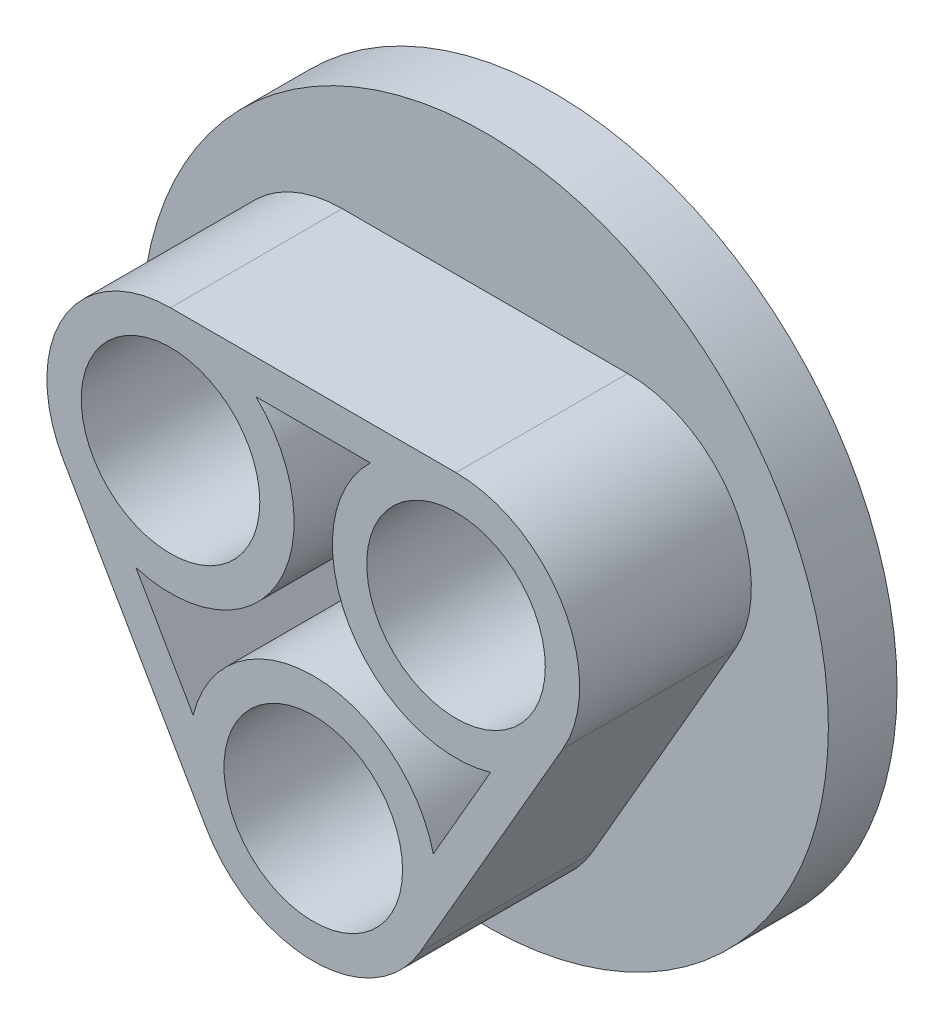
ISO-10303-21;
HEADER;
FILE_DESCRIPTION(('STEP AP214'),'2;1');
FILE_NAME('part.step','',(''),(''),'','','');
FILE_SCHEMA(('AUTOMOTIVE_DESIGN { 1 0 10303 214 1 1 1 1 }'));
ENDSEC;
DATA;
#1=APPLICATION_CONTEXT('core data for automotive mechanical design processes');
#2=APPLICATION_PROTOCOL_DEFINITION('international standard','automotive_design',2000,#1);
#3=PRODUCT_CONTEXT('',#1,'mechanical');
#4=PRODUCT('Part','Part','',(#3));
#5=PRODUCT_RELATED_PRODUCT_CATEGORY('part','',(#4));
#6=PRODUCT_DEFINITION_FORMATION('','',#4);
#7=PRODUCT_DEFINITION_CONTEXT('part definition',#1,'design');
#8=PRODUCT_DEFINITION('design','',#6,#7);
#9=PRODUCT_DEFINITION_SHAPE('','',#8);
#10=(LENGTH_UNIT() NAMED_UNIT(*) SI_UNIT(.MILLI.,.METRE.));
#11=(NAMED_UNIT(*) PLANE_ANGLE_UNIT() SI_UNIT($,.RADIAN.));
#12=(NAMED_UNIT(*) SI_UNIT($,.STERADIAN.) SOLID_ANGLE_UNIT());
#13=UNCERTAINTY_MEASURE_WITH_UNIT(LENGTH_MEASURE(1.E-05),#10,'distance_accuracy_value','');
#14=(GEOMETRIC_REPRESENTATION_CONTEXT(3) GLOBAL_UNCERTAINTY_ASSIGNED_CONTEXT((#13)) GLOBAL_UNIT_ASSIGNED_CONTEXT((#10,
#11,#12)) REPRESENTATION_CONTEXT('',''));
#15=CARTESIAN_POINT('',(0.,0.,0.));
#16=DIRECTION('',(0.,0.,1.));
#17=DIRECTION('',(1.,0.,0.));
#18=AXIS2_PLACEMENT_3D('',#15,#16,#17);
#19=CARTESIAN_POINT('',(0.,0.,10.));
#20=DIRECTION('',(0.,0.,1.));
#21=DIRECTION('',(1.,0.,0.));
#22=AXIS2_PLACEMENT_3D('',#19,#20,#21);
#23=PLANE('',#22);
#24=CARTESIAN_POINT('',(0.,0.,10.));
#25=DIRECTION('',(0.,0.,1.));
#26=DIRECTION('',(1.,0.,0.));
#27=AXIS2_PLACEMENT_3D('',#24,#25,#26);
#28=CIRCLE('',#27,50.);
#29=CARTESIAN_POINT('',(50.,0.,10.));
#30=VERTEX_POINT('',#29);
#31=EDGE_CURVE('E244',#30,#30,#28,.T.);
#32=ORIENTED_EDGE('',*,*,#31,.T.);
#33=EDGE_LOOP('',(#32));
#34=FACE_BOUND('',#33,.T.);
#35=DIRECTION('',(-0.499999999999999,-0.866025403784439,0.));
#36=VECTOR('',#35,1.);
#37=CARTESIAN_POINT('',(25.9807621135332,-15.,10.));
#38=LINE('',#37,#36);
#39=CARTESIAN_POINT('',(36.3730669589464,3.00000000000004,10.));
#40=VERTEX_POINT('',#39);
#41=CARTESIAN_POINT('',(15.5884572681199,-33.,10.));
#42=VERTEX_POINT('',#41);
#43=EDGE_CURVE('E212',#40,#42,#38,.T.);
#44=ORIENTED_EDGE('',*,*,#43,.T.);
#45=CARTESIAN_POINT('',(0.,-24.,10.));
#46=DIRECTION('',(0.,0.,1.));
#47=DIRECTION('',(1.,0.,0.));
#48=AXIS2_PLACEMENT_3D('',#45,#46,#47);
#49=CIRCLE('',#48,18.);
#50=CARTESIAN_POINT('',(-15.5884572681199,-33.,10.));
#51=VERTEX_POINT('',#50);
#52=EDGE_CURVE('E204',#51,#42,#49,.T.);
#53=ORIENTED_EDGE('',*,*,#52,.F.);
#54=DIRECTION('',(0.5,-0.866025403784439,0.));
#55=VECTOR('',#54,1.);
#56=CARTESIAN_POINT('',(-25.9807621135332,-15.,10.));
#57=LINE('',#56,#55);
#58=CARTESIAN_POINT('',(-36.3730669589464,3.00000000000003,10.));
#59=VERTEX_POINT('',#58);
#60=EDGE_CURVE('E163',#59,#51,#57,.T.);
#61=ORIENTED_EDGE('',*,*,#60,.F.);
#62=CARTESIAN_POINT('',(-20.7846096908265,12.,10.));
#63=DIRECTION('',(0.,0.,1.));
#64=DIRECTION('',(1.,0.,0.));
#65=AXIS2_PLACEMENT_3D('',#62,#63,#64);
#66=CIRCLE('',#65,18.);
#67=CARTESIAN_POINT('',(-20.7846096908265,30.,10.));
#68=VERTEX_POINT('',#67);
#69=EDGE_CURVE('E167',#68,#59,#66,.T.);
#70=ORIENTED_EDGE('',*,*,#69,.F.);
#71=DIRECTION('',(1.,0.,0.));
#72=VECTOR('',#71,1.);
#73=CARTESIAN_POINT('',(0.,30.,10.));
#74=LINE('',#73,#72);
#75=CARTESIAN_POINT('',(20.7846096908265,30.,10.));
#76=VERTEX_POINT('',#75);
#77=EDGE_CURVE('E220',#68,#76,#74,.T.);
#78=ORIENTED_EDGE('',*,*,#77,.T.);
#79=CARTESIAN_POINT('',(20.7846096908265,12.,10.));
#80=DIRECTION('',(0.,0.,1.));
#81=DIRECTION('',(1.,0.,0.));
#82=AXIS2_PLACEMENT_3D('',#79,#80,#81);
#83=CIRCLE('',#82,18.);
#84=EDGE_CURVE('E213',#40,#76,#83,.T.);
#85=ORIENTED_EDGE('',*,*,#84,.F.);
#86=EDGE_LOOP('',(#44,#53,#61,#70,#78,#85));
#87=FACE_BOUND('',#86,.T.);
#88=ADVANCED_FACE('F50',(#34,#87),#23,.T.);
#89=CARTESIAN_POINT('',(0.,0.,10.));
#90=DIRECTION('',(0.,0.,-1.));
#91=DIRECTION('',(-1.,0.,0.));
#92=AXIS2_PLACEMENT_3D('',#89,#90,#91);
#93=CYLINDRICAL_SURFACE('',#92,50.);
#94=ORIENTED_EDGE('',*,*,#31,.F.);
#95=EDGE_LOOP('',(#94));
#96=FACE_BOUND('',#95,.T.);
#97=CARTESIAN_POINT('',(0.,0.,0.));
#98=DIRECTION('',(0.,0.,1.));
#99=DIRECTION('',(1.,0.,0.));
#100=AXIS2_PLACEMENT_3D('',#97,#98,#99);
#101=CIRCLE('',#100,50.);
#102=CARTESIAN_POINT('',(50.,0.,0.));
#103=VERTEX_POINT('',#102);
#104=EDGE_CURVE('E233',#103,#103,#101,.T.);
#105=ORIENTED_EDGE('',*,*,#104,.T.);
#106=EDGE_LOOP('',(#105));
#107=FACE_BOUND('',#106,.T.);
#108=ADVANCED_FACE('F47',(#96,#107),#93,.T.);
#109=CARTESIAN_POINT('',(0.,0.,0.));
#110=DIRECTION('',(0.,0.,1.));
#111=DIRECTION('',(1.,0.,0.));
#112=AXIS2_PLACEMENT_3D('',#109,#110,#111);
#113=PLANE('',#112);
#114=CARTESIAN_POINT('',(0.,0.,0.));
#115=DIRECTION('',(0.,0.,-1.));
#116=DIRECTION('',(-1.,0.,0.));
#117=AXIS2_PLACEMENT_3D('',#114,#115,#116);
#118=CIRCLE('',#117,45.);
#119=CARTESIAN_POINT('',(-45.,0.,0.));
#120=VERTEX_POINT('',#119);
#121=EDGE_CURVE('E166',#120,#120,#118,.T.);
#122=ORIENTED_EDGE('',*,*,#121,.F.);
#123=EDGE_LOOP('',(#122));
#124=FACE_BOUND('',#123,.T.);
#125=ORIENTED_EDGE('',*,*,#104,.F.);
#126=EDGE_LOOP('',(#125));
#127=FACE_BOUND('',#126,.T.);
#128=ADVANCED_FACE('F296',(#124,#127),#113,.F.);
#129=CARTESIAN_POINT('',(0.,-24.,35.));
#130=DIRECTION('',(0.,0.,-1.));
#131=DIRECTION('',(-1.,0.,0.));
#132=AXIS2_PLACEMENT_3D('',#129,#130,#131);
#133=CYLINDRICAL_SURFACE('',#132,18.);
#134=ORIENTED_EDGE('',*,*,#52,.T.);
#135=DIRECTION('',(0.,0.,-1.));
#136=VECTOR('',#135,1.);
#137=CARTESIAN_POINT('',(15.5884572681199,-33.,35.));
#138=LINE('',#137,#136);
#139=CARTESIAN_POINT('',(15.5884572681199,-33.,35.));
#140=VERTEX_POINT('',#139);
#141=EDGE_CURVE('E228',#140,#42,#138,.T.);
#142=ORIENTED_EDGE('',*,*,#141,.F.);
#143=CARTESIAN_POINT('',(0.,-24.,35.));
#144=DIRECTION('',(0.,0.,1.));
#145=DIRECTION('',(1.,0.,0.));
#146=AXIS2_PLACEMENT_3D('',#143,#144,#145);
#147=CIRCLE('',#146,18.);
#148=CARTESIAN_POINT('',(-15.5884572681199,-33.,35.));
#149=VERTEX_POINT('',#148);
#150=EDGE_CURVE('E160',#149,#140,#147,.T.);
#151=ORIENTED_EDGE('',*,*,#150,.F.);
#152=DIRECTION('',(0.,0.,-1.));
#153=VECTOR('',#152,1.);
#154=CARTESIAN_POINT('',(-15.5884572681199,-33.,35.));
#155=LINE('',#154,#153);
#156=EDGE_CURVE('E148',#149,#51,#155,.T.);
#157=ORIENTED_EDGE('',*,*,#156,.T.);
#158=EDGE_LOOP('',(#134,#142,#151,#157));
#159=FACE_BOUND('',#158,.T.);
#160=ADVANCED_FACE('F297',(#159),#133,.T.);
#161=CARTESIAN_POINT('',(25.9807621135332,-15.,35.));
#162=DIRECTION('',(0.866025403784439,-0.499999999999999,0.));
#163=DIRECTION('',(0.499999999999999,0.866025403784439,0.));
#164=AXIS2_PLACEMENT_3D('',#161,#162,#163);
#165=PLANE('',#164);
#166=ORIENTED_EDGE('',*,*,#43,.F.);
#167=DIRECTION('',(0.,0.,-1.));
#168=VECTOR('',#167,1.);
#169=CARTESIAN_POINT('',(36.3730669589464,3.00000000000004,35.));
#170=LINE('',#169,#168);
#171=CARTESIAN_POINT('',(36.3730669589464,3.00000000000004,35.));
#172=VERTEX_POINT('',#171);
#173=EDGE_CURVE('E226',#172,#40,#170,.T.);
#174=ORIENTED_EDGE('',*,*,#173,.F.);
#175=DIRECTION('',(-0.499999999999999,-0.866025403784439,0.));
#176=VECTOR('',#175,1.);
#177=CARTESIAN_POINT('',(25.9807621135332,-15.,35.));
#178=LINE('',#177,#176);
#179=EDGE_CURVE('E187',#172,#140,#178,.T.);
#180=ORIENTED_EDGE('',*,*,#179,.T.);
#181=ORIENTED_EDGE('',*,*,#141,.T.);
#182=EDGE_LOOP('',(#166,#174,#180,#181));
#183=FACE_BOUND('',#182,.T.);
#184=ADVANCED_FACE('F325',(#183),#165,.T.);
#185=CARTESIAN_POINT('',(20.7846096908265,12.,35.));
#186=DIRECTION('',(0.,0.,-1.));
#187=DIRECTION('',(-1.,0.,0.));
#188=AXIS2_PLACEMENT_3D('',#185,#186,#187);
#189=CYLINDRICAL_SURFACE('',#188,18.);
#190=ORIENTED_EDGE('',*,*,#84,.T.);
#191=DIRECTION('',(0.,0.,-1.));
#192=VECTOR('',#191,1.);
#193=CARTESIAN_POINT('',(20.7846096908265,30.,35.));
#194=LINE('',#193,#192);
#195=CARTESIAN_POINT('',(20.7846096908265,30.,35.));
#196=VERTEX_POINT('',#195);
#197=EDGE_CURVE('E223',#196,#76,#194,.T.);
#198=ORIENTED_EDGE('',*,*,#197,.F.);
#199=CARTESIAN_POINT('',(20.7846096908265,12.,35.));
#200=DIRECTION('',(0.,0.,1.));
#201=DIRECTION('',(1.,0.,0.));
#202=AXIS2_PLACEMENT_3D('',#199,#200,#201);
#203=CIRCLE('',#202,18.);
#204=EDGE_CURVE('E182',#172,#196,#203,.T.);
#205=ORIENTED_EDGE('',*,*,#204,.F.);
#206=ORIENTED_EDGE('',*,*,#173,.T.);
#207=EDGE_LOOP('',(#190,#198,#205,#206));
#208=FACE_BOUND('',#207,.T.);
#209=ADVANCED_FACE('F337',(#208),#189,.T.);
#210=CARTESIAN_POINT('',(0.,30.,35.));
#211=DIRECTION('',(0.,1.,0.));
#212=DIRECTION('',(-1.,0.,0.));
#213=AXIS2_PLACEMENT_3D('',#210,#211,#212);
#214=PLANE('',#213);
#215=ORIENTED_EDGE('',*,*,#77,.F.);
#216=DIRECTION('',(0.,0.,-1.));
#217=VECTOR('',#216,1.);
#218=CARTESIAN_POINT('',(-20.7846096908265,30.,35.));
#219=LINE('',#218,#217);
#220=CARTESIAN_POINT('',(-20.7846096908265,30.,35.));
#221=VERTEX_POINT('',#220);
#222=EDGE_CURVE('E224',#221,#68,#219,.T.);
#223=ORIENTED_EDGE('',*,*,#222,.F.);
#224=DIRECTION('',(1.,0.,0.));
#225=VECTOR('',#224,1.);
#226=CARTESIAN_POINT('',(0.,30.,35.));
#227=LINE('',#226,#225);
#228=EDGE_CURVE('E191',#221,#196,#227,.T.);
#229=ORIENTED_EDGE('',*,*,#228,.T.);
#230=ORIENTED_EDGE('',*,*,#197,.T.);
#231=EDGE_LOOP('',(#215,#223,#229,#230));
#232=FACE_BOUND('',#231,.T.);
#233=ADVANCED_FACE('F336',(#232),#214,.T.);
#234=CARTESIAN_POINT('',(-20.7846096908265,12.,35.));
#235=DIRECTION('',(0.,0.,-1.));
#236=DIRECTION('',(-1.,0.,0.));
#237=AXIS2_PLACEMENT_3D('',#234,#235,#236);
#238=CYLINDRICAL_SURFACE('',#237,18.);
#239=ORIENTED_EDGE('',*,*,#69,.T.);
#240=DIRECTION('',(0.,0.,-1.));
#241=VECTOR('',#240,1.);
#242=CARTESIAN_POINT('',(-36.3730669589464,3.00000000000003,35.));
#243=LINE('',#242,#241);
#244=CARTESIAN_POINT('',(-36.3730669589464,3.00000000000003,35.));
#245=VERTEX_POINT('',#244);
#246=EDGE_CURVE('E67',#245,#59,#243,.T.);
#247=ORIENTED_EDGE('',*,*,#246,.F.);
#248=CARTESIAN_POINT('',(-20.7846096908265,12.,35.));
#249=DIRECTION('',(0.,0.,1.));
#250=DIRECTION('',(1.,0.,0.));
#251=AXIS2_PLACEMENT_3D('',#248,#249,#250);
#252=CIRCLE('',#251,18.);
#253=EDGE_CURVE('E178',#221,#245,#252,.T.);
#254=ORIENTED_EDGE('',*,*,#253,.F.);
#255=ORIENTED_EDGE('',*,*,#222,.T.);
#256=EDGE_LOOP('',(#239,#247,#254,#255));
#257=FACE_BOUND('',#256,.T.);
#258=ADVANCED_FACE('F334',(#257),#238,.T.);
#259=CARTESIAN_POINT('',(21.650635094611,-12.5,35.));
#260=DIRECTION('',(-0.866025403784439,0.499999999999999,0.));
#261=DIRECTION('',(-0.499999999999999,-0.866025403784439,0.));
#262=AXIS2_PLACEMENT_3D('',#259,#260,#261);
#263=PLANE('',#262);
#264=DIRECTION('',(0.499999999999999,0.866025403784439,0.));
#265=VECTOR('',#264,1.);
#266=CARTESIAN_POINT('',(21.650635094611,-12.5,10.));
#267=LINE('',#266,#265);
#268=CARTESIAN_POINT('',(17.4832800481921,-19.7180706735761,10.));
#269=VERTEX_POINT('',#268);
#270=CARTESIAN_POINT('',(25.8179901410299,-5.28192932642387,10.));
#271=VERTEX_POINT('',#270);
#272=EDGE_CURVE('E141',#269,#271,#267,.T.);
#273=ORIENTED_EDGE('',*,*,#272,.F.);
#274=DIRECTION('',(0.,0.,-1.));
#275=VECTOR('',#274,1.);
#276=CARTESIAN_POINT('',(17.4832800481921,-19.7180706735761,35.));
#277=LINE('',#276,#275);
#278=CARTESIAN_POINT('',(17.4832800481921,-19.7180706735761,35.));
#279=VERTEX_POINT('',#278);
#280=EDGE_CURVE('E140',#279,#269,#277,.T.);
#281=ORIENTED_EDGE('',*,*,#280,.F.);
#282=DIRECTION('',(0.499999999999999,0.866025403784439,0.));
#283=VECTOR('',#282,1.);
#284=CARTESIAN_POINT('',(21.650635094611,-12.5,35.));
#285=LINE('',#284,#283);
#286=CARTESIAN_POINT('',(25.8179901410299,-5.28192932642387,35.));
#287=VERTEX_POINT('',#286);
#288=EDGE_CURVE('E143',#279,#287,#285,.T.);
#289=ORIENTED_EDGE('',*,*,#288,.T.);
#290=DIRECTION('',(0.,0.,-1.));
#291=VECTOR('',#290,1.);
#292=CARTESIAN_POINT('',(25.8179901410299,-5.28192932642387,35.));
#293=LINE('',#292,#291);
#294=EDGE_CURVE('E196',#287,#271,#293,.T.);
#295=ORIENTED_EDGE('',*,*,#294,.T.);
#296=EDGE_LOOP('',(#273,#281,#289,#295));
#297=FACE_BOUND('',#296,.T.);
#298=ADVANCED_FACE('F139',(#297),#263,.T.);
#299=CARTESIAN_POINT('',(-17.4832800481921,-19.7180706735761,10.));
#300=VERTEX_POINT('',#299);
#301=EDGE_CURVE('E199',#269,#300,#49,.T.);
#302=ORIENTED_EDGE('',*,*,#301,.T.);
#303=DIRECTION('',(0.,0.,-1.));
#304=VECTOR('',#303,1.);
#305=CARTESIAN_POINT('',(-17.4832800481921,-19.7180706735761,35.));
#306=LINE('',#305,#304);
#307=CARTESIAN_POINT('',(-17.4832800481921,-19.7180706735761,35.));
#308=VERTEX_POINT('',#307);
#309=EDGE_CURVE('E150',#308,#300,#306,.T.);
#310=ORIENTED_EDGE('',*,*,#309,.F.);
#311=EDGE_CURVE('E147',#279,#308,#147,.T.);
#312=ORIENTED_EDGE('',*,*,#311,.F.);
#313=ORIENTED_EDGE('',*,*,#280,.T.);
#314=EDGE_LOOP('',(#302,#310,#312,#313));
#315=FACE_BOUND('',#314,.T.);
#316=ADVANCED_FACE('F151',(#315),#133,.T.);
#317=CARTESIAN_POINT('',(-21.650635094611,-12.5,35.));
#318=DIRECTION('',(-0.866025403784439,-0.5,0.));
#319=DIRECTION('',(0.5,-0.866025403784439,0.));
#320=AXIS2_PLACEMENT_3D('',#317,#318,#319);
#321=PLANE('',#320);
#322=DIRECTION('',(-0.5,0.866025403784439,0.));
#323=VECTOR('',#322,1.);
#324=CARTESIAN_POINT('',(-21.650635094611,-12.5,10.));
#325=LINE('',#324,#323);
#326=CARTESIAN_POINT('',(-25.8179901410299,-5.28192932642388,10.));
#327=VERTEX_POINT('',#326);
#328=EDGE_CURVE('E201',#300,#327,#325,.T.);
#329=ORIENTED_EDGE('',*,*,#328,.T.);
#330=DIRECTION('',(0.,0.,-1.));
#331=VECTOR('',#330,1.);
#332=CARTESIAN_POINT('',(-25.8179901410299,-5.28192932642388,35.));
#333=LINE('',#332,#331);
#334=CARTESIAN_POINT('',(-25.8179901410299,-5.28192932642388,35.));
#335=VERTEX_POINT('',#334);
#336=EDGE_CURVE('E240',#335,#327,#333,.T.);
#337=ORIENTED_EDGE('',*,*,#336,.F.);
#338=DIRECTION('',(-0.5,0.866025403784439,0.));
#339=VECTOR('',#338,1.);
#340=CARTESIAN_POINT('',(-21.650635094611,-12.5,35.));
#341=LINE('',#340,#339);
#342=EDGE_CURVE('E154',#308,#335,#341,.T.);
#343=ORIENTED_EDGE('',*,*,#342,.F.);
#344=ORIENTED_EDGE('',*,*,#309,.T.);
#345=EDGE_LOOP('',(#329,#337,#343,#344));
#346=FACE_BOUND('',#345,.T.);
#347=ADVANCED_FACE('F382',(#346),#321,.F.);
#348=CARTESIAN_POINT('',(-8.33471009283779,25.,10.));
#349=VERTEX_POINT('',#348);
#350=EDGE_CURVE('E206',#327,#349,#66,.T.);
#351=ORIENTED_EDGE('',*,*,#350,.T.);
#352=DIRECTION('',(0.,0.,-1.));
#353=VECTOR('',#352,1.);
#354=CARTESIAN_POINT('',(-8.33471009283779,25.,35.));
#355=LINE('',#354,#353);
#356=CARTESIAN_POINT('',(-8.33471009283779,25.,35.));
#357=VERTEX_POINT('',#356);
#358=EDGE_CURVE('E232',#357,#349,#355,.T.);
#359=ORIENTED_EDGE('',*,*,#358,.F.);
#360=EDGE_CURVE('E175',#335,#357,#252,.T.);
#361=ORIENTED_EDGE('',*,*,#360,.F.);
#362=ORIENTED_EDGE('',*,*,#336,.T.);
#363=EDGE_LOOP('',(#351,#359,#361,#362));
#364=FACE_BOUND('',#363,.T.);
#365=ADVANCED_FACE('F359',(#364),#238,.T.);
#366=CARTESIAN_POINT('',(0.,25.,35.));
#367=DIRECTION('',(0.,-1.,0.));
#368=DIRECTION('',(0.,0.,-1.));
#369=AXIS2_PLACEMENT_3D('',#366,#367,#368);
#370=PLANE('',#369);
#371=DIRECTION('',(-1.,0.,0.));
#372=VECTOR('',#371,1.);
#373=CARTESIAN_POINT('',(0.,25.,10.));
#374=LINE('',#373,#372);
#375=CARTESIAN_POINT('',(8.33471009283778,25.,10.));
#376=VERTEX_POINT('',#375);
#377=EDGE_CURVE('E61',#376,#349,#374,.T.);
#378=ORIENTED_EDGE('',*,*,#377,.F.);
#379=DIRECTION('',(0.,0.,-1.));
#380=VECTOR('',#379,1.);
#381=CARTESIAN_POINT('',(8.33471009283778,25.,35.));
#382=LINE('',#381,#380);
#383=CARTESIAN_POINT('',(8.33471009283778,25.,35.));
#384=VERTEX_POINT('',#383);
#385=EDGE_CURVE('E231',#384,#376,#382,.T.);
#386=ORIENTED_EDGE('',*,*,#385,.F.);
#387=DIRECTION('',(-1.,0.,0.));
#388=VECTOR('',#387,1.);
#389=CARTESIAN_POINT('',(0.,25.,35.));
#390=LINE('',#389,#388);
#391=EDGE_CURVE('E172',#384,#357,#390,.T.);
#392=ORIENTED_EDGE('',*,*,#391,.T.);
#393=ORIENTED_EDGE('',*,*,#358,.T.);
#394=EDGE_LOOP('',(#378,#386,#392,#393));
#395=FACE_BOUND('',#394,.T.);
#396=ADVANCED_FACE('F375',(#395),#370,.T.);
#397=CARTESIAN_POINT('',(-20.7846096908265,12.,35.));
#398=DIRECTION('',(0.,0.,-1.));
#399=DIRECTION('',(-1.,0.,0.));
#400=AXIS2_PLACEMENT_3D('',#397,#398,#399);
#401=CYLINDRICAL_SURFACE('',#400,13.);
#402=CARTESIAN_POINT('',(-20.7846096908265,12.,35.));
#403=DIRECTION('',(0.,0.,1.));
#404=DIRECTION('',(1.,0.,0.));
#405=AXIS2_PLACEMENT_3D('',#402,#403,#404);
#406=CIRCLE('',#405,13.);
#407=CARTESIAN_POINT('',(-7.78460969082652,12.,35.));
#408=VERTEX_POINT('',#407);
#409=EDGE_CURVE('E186',#408,#408,#406,.T.);
#410=ORIENTED_EDGE('',*,*,#409,.T.);
#411=EDGE_LOOP('',(#410));
#412=FACE_BOUND('',#411,.T.);
#413=CARTESIAN_POINT('',(-20.7846096908265,12.,10.));
#414=DIRECTION('',(0.,0.,1.));
#415=DIRECTION('',(1.,0.,0.));
#416=AXIS2_PLACEMENT_3D('',#413,#414,#415);
#417=CIRCLE('',#416,13.);
#418=CARTESIAN_POINT('',(-7.78460969082652,12.,10.));
#419=VERTEX_POINT('',#418);
#420=EDGE_CURVE('E252',#419,#419,#417,.F.);
#421=ORIENTED_EDGE('',*,*,#420,.T.);
#422=EDGE_LOOP('',(#421));
#423=FACE_BOUND('',#422,.T.);
#424=ADVANCED_FACE('F366',(#412,#423),#401,.F.);
#425=CARTESIAN_POINT('',(20.7846096908265,12.,35.));
#426=DIRECTION('',(0.,0.,-1.));
#427=DIRECTION('',(-1.,0.,0.));
#428=AXIS2_PLACEMENT_3D('',#425,#426,#427);
#429=CYLINDRICAL_SURFACE('',#428,13.);
#430=CARTESIAN_POINT('',(20.7846096908265,12.,35.));
#431=DIRECTION('',(0.,0.,1.));
#432=DIRECTION('',(1.,0.,0.));
#433=AXIS2_PLACEMENT_3D('',#430,#431,#432);
#434=CIRCLE('',#433,13.);
#435=CARTESIAN_POINT('',(33.7846096908265,12.,35.));
#436=VERTEX_POINT('',#435);
#437=EDGE_CURVE('E184',#436,#436,#434,.T.);
#438=ORIENTED_EDGE('',*,*,#437,.T.);
#439=EDGE_LOOP('',(#438));
#440=FACE_BOUND('',#439,.T.);
#441=CARTESIAN_POINT('',(20.7846096908265,12.,10.));
#442=DIRECTION('',(0.,0.,1.));
#443=DIRECTION('',(1.,0.,0.));
#444=AXIS2_PLACEMENT_3D('',#441,#442,#443);
#445=CIRCLE('',#444,13.);
#446=CARTESIAN_POINT('',(33.7846096908265,12.,10.));
#447=VERTEX_POINT('',#446);
#448=EDGE_CURVE('E249',#447,#447,#445,.F.);
#449=ORIENTED_EDGE('',*,*,#448,.T.);
#450=EDGE_LOOP('',(#449));
#451=FACE_BOUND('',#450,.T.);
#452=ADVANCED_FACE('F371',(#440,#451),#429,.F.);
#453=CARTESIAN_POINT('',(0.,-24.,35.));
#454=DIRECTION('',(0.,0.,-1.));
#455=DIRECTION('',(-1.,0.,0.));
#456=AXIS2_PLACEMENT_3D('',#453,#454,#455);
#457=CYLINDRICAL_SURFACE('',#456,13.);
#458=CARTESIAN_POINT('',(0.,-24.,35.));
#459=DIRECTION('',(0.,0.,1.));
#460=DIRECTION('',(1.,0.,0.));
#461=AXIS2_PLACEMENT_3D('',#458,#459,#460);
#462=CIRCLE('',#461,13.);
#463=CARTESIAN_POINT('',(13.,-24.,35.));
#464=VERTEX_POINT('',#463);
#465=EDGE_CURVE('E177',#464,#464,#462,.T.);
#466=ORIENTED_EDGE('',*,*,#465,.T.);
#467=EDGE_LOOP('',(#466));
#468=FACE_BOUND('',#467,.T.);
#469=CARTESIAN_POINT('',(0.,-24.,10.));
#470=DIRECTION('',(0.,0.,1.));
#471=DIRECTION('',(1.,0.,0.));
#472=AXIS2_PLACEMENT_3D('',#469,#470,#471);
#473=CIRCLE('',#472,13.);
#474=CARTESIAN_POINT('',(13.,-24.,10.));
#475=VERTEX_POINT('',#474);
#476=EDGE_CURVE('E243',#475,#475,#473,.F.);
#477=ORIENTED_EDGE('',*,*,#476,.T.);
#478=EDGE_LOOP('',(#477));
#479=FACE_BOUND('',#478,.T.);
#480=ADVANCED_FACE('F376',(#468,#479),#457,.F.);
#481=EDGE_CURVE('E209',#376,#271,#83,.T.);
#482=ORIENTED_EDGE('',*,*,#481,.T.);
#483=ORIENTED_EDGE('',*,*,#294,.F.);
#484=EDGE_CURVE('E165',#384,#287,#203,.T.);
#485=ORIENTED_EDGE('',*,*,#484,.F.);
#486=ORIENTED_EDGE('',*,*,#385,.T.);
#487=EDGE_LOOP('',(#482,#483,#485,#486));
#488=FACE_BOUND('',#487,.T.);
#489=ADVANCED_FACE('F351',(#488),#189,.T.);
#490=CARTESIAN_POINT('',(-25.9807621135332,-15.,35.));
#491=DIRECTION('',(0.866025403784439,0.5,0.));
#492=DIRECTION('',(-0.5,0.866025403784439,0.));
#493=AXIS2_PLACEMENT_3D('',#490,#491,#492);
#494=PLANE('',#493);
#495=ORIENTED_EDGE('',*,*,#60,.T.);
#496=ORIENTED_EDGE('',*,*,#156,.F.);
#497=DIRECTION('',(0.5,-0.866025403784439,0.));
#498=VECTOR('',#497,1.);
#499=CARTESIAN_POINT('',(-25.9807621135332,-15.,35.));
#500=LINE('',#499,#498);
#501=EDGE_CURVE('E198',#245,#149,#500,.T.);
#502=ORIENTED_EDGE('',*,*,#501,.F.);
#503=ORIENTED_EDGE('',*,*,#246,.T.);
#504=EDGE_LOOP('',(#495,#496,#502,#503));
#505=FACE_BOUND('',#504,.T.);
#506=ADVANCED_FACE('F328',(#505),#494,.F.);
#507=CARTESIAN_POINT('',(0.,0.,35.));
#508=DIRECTION('',(0.,0.,1.));
#509=DIRECTION('',(1.,0.,0.));
#510=AXIS2_PLACEMENT_3D('',#507,#508,#509);
#511=PLANE('',#510);
#512=ORIENTED_EDGE('',*,*,#501,.T.);
#513=ORIENTED_EDGE('',*,*,#150,.T.);
#514=ORIENTED_EDGE('',*,*,#179,.F.);
#515=ORIENTED_EDGE('',*,*,#204,.T.);
#516=ORIENTED_EDGE('',*,*,#228,.F.);
#517=ORIENTED_EDGE('',*,*,#253,.T.);
#518=EDGE_LOOP('',(#512,#513,#514,#515,#516,#517));
#519=FACE_BOUND('',#518,.T.);
#520=ORIENTED_EDGE('',*,*,#311,.T.);
#521=ORIENTED_EDGE('',*,*,#342,.T.);
#522=ORIENTED_EDGE('',*,*,#360,.T.);
#523=ORIENTED_EDGE('',*,*,#391,.F.);
#524=ORIENTED_EDGE('',*,*,#484,.T.);
#525=ORIENTED_EDGE('',*,*,#288,.F.);
#526=EDGE_LOOP('',(#520,#521,#522,#523,#524,#525));
#527=FACE_BOUND('',#526,.T.);
#528=ORIENTED_EDGE('',*,*,#437,.F.);
#529=EDGE_LOOP('',(#528));
#530=FACE_BOUND('',#529,.T.);
#531=ORIENTED_EDGE('',*,*,#409,.F.);
#532=EDGE_LOOP('',(#531));
#533=FACE_BOUND('',#532,.T.);
#534=ORIENTED_EDGE('',*,*,#465,.F.);
#535=EDGE_LOOP('',(#534));
#536=FACE_BOUND('',#535,.T.);
#537=ADVANCED_FACE('F158',(#519,#527,#530,#533,#536),#511,.T.);
#538=ORIENTED_EDGE('',*,*,#272,.T.);
#539=ORIENTED_EDGE('',*,*,#481,.F.);
#540=ORIENTED_EDGE('',*,*,#377,.T.);
#541=ORIENTED_EDGE('',*,*,#350,.F.);
#542=ORIENTED_EDGE('',*,*,#328,.F.);
#543=ORIENTED_EDGE('',*,*,#301,.F.);
#544=EDGE_LOOP('',(#538,#539,#540,#541,#542,#543));
#545=FACE_BOUND('',#544,.T.);
#546=ADVANCED_FACE('F313',(#545),#23,.T.);
#547=ORIENTED_EDGE('',*,*,#476,.F.);
#548=EDGE_LOOP('',(#547));
#549=FACE_BOUND('',#548,.T.);
#550=ADVANCED_FACE('F315',(#549),#23,.T.);
#551=ORIENTED_EDGE('',*,*,#448,.F.);
#552=EDGE_LOOP('',(#551));
#553=FACE_BOUND('',#552,.T.);
#554=ADVANCED_FACE('F421',(#553),#23,.T.);
#555=ORIENTED_EDGE('',*,*,#420,.F.);
#556=EDGE_LOOP('',(#555));
#557=FACE_BOUND('',#556,.T.);
#558=ADVANCED_FACE('F348',(#557),#23,.T.);
#559=CARTESIAN_POINT('',(0.,0.,5.));
#560=DIRECTION('',(0.,0.,-1.));
#561=DIRECTION('',(-1.,0.,0.));
#562=AXIS2_PLACEMENT_3D('',#559,#560,#561);
#563=CYLINDRICAL_SURFACE('',#562,45.);
#564=CARTESIAN_POINT('',(0.,0.,5.));
#565=DIRECTION('',(0.,0.,-1.));
#566=DIRECTION('',(-1.,0.,0.));
#567=AXIS2_PLACEMENT_3D('',#564,#565,#566);
#568=CIRCLE('',#567,45.);
#569=CARTESIAN_POINT('',(-45.,0.,5.));
#570=VERTEX_POINT('',#569);
#571=EDGE_CURVE('E203',#570,#570,#568,.T.);
#572=ORIENTED_EDGE('',*,*,#571,.F.);
#573=EDGE_LOOP('',(#572));
#574=FACE_BOUND('',#573,.T.);
#575=ORIENTED_EDGE('',*,*,#121,.T.);
#576=EDGE_LOOP('',(#575));
#577=FACE_BOUND('',#576,.T.);
#578=ADVANCED_FACE('F293',(#574,#577),#563,.F.);
#579=CARTESIAN_POINT('',(0.,0.,5.));
#580=DIRECTION('',(0.,0.,-1.));
#581=DIRECTION('',(-1.,0.,0.));
#582=AXIS2_PLACEMENT_3D('',#579,#580,#581);
#583=PLANE('',#582);
#584=CARTESIAN_POINT('',(0.,-24.,5.));
#585=DIRECTION('',(0.,0.,-1.));
#586=DIRECTION('',(-1.,0.,0.));
#587=AXIS2_PLACEMENT_3D('',#584,#585,#586);
#588=CIRCLE('',#587,18.);
#589=CARTESIAN_POINT('',(-18.,-24.,5.));
#590=VERTEX_POINT('',#589);
#591=EDGE_CURVE('E11',#590,#590,#588,.T.);
#592=ORIENTED_EDGE('',*,*,#591,.F.);
#593=EDGE_LOOP('',(#592));
#594=FACE_BOUND('',#593,.T.);
#595=CARTESIAN_POINT('',(-20.7846096908265,12.,5.));
#596=DIRECTION('',(0.,0.,-1.));
#597=DIRECTION('',(-1.,0.,0.));
#598=AXIS2_PLACEMENT_3D('',#595,#596,#597);
#599=CIRCLE('',#598,18.);
#600=CARTESIAN_POINT('',(-38.7846096908265,12.,5.));
#601=VERTEX_POINT('',#600);
#602=EDGE_CURVE('E54',#601,#601,#599,.T.);
#603=ORIENTED_EDGE('',*,*,#602,.F.);
#604=EDGE_LOOP('',(#603));
#605=FACE_BOUND('',#604,.T.);
#606=CARTESIAN_POINT('',(20.7846096908265,12.,5.));
#607=DIRECTION('',(0.,0.,-1.));
#608=DIRECTION('',(-1.,0.,0.));
#609=AXIS2_PLACEMENT_3D('',#606,#607,#608);
#610=CIRCLE('',#609,18.);
#611=CARTESIAN_POINT('',(2.78460969082652,12.,5.));
#612=VERTEX_POINT('',#611);
#613=EDGE_CURVE('E254',#612,#612,#610,.T.);
#614=ORIENTED_EDGE('',*,*,#613,.F.);
#615=EDGE_LOOP('',(#614));
#616=FACE_BOUND('',#615,.T.);
#617=ORIENTED_EDGE('',*,*,#571,.T.);
#618=EDGE_LOOP('',(#617));
#619=FACE_BOUND('',#618,.T.);
#620=ADVANCED_FACE('F436',(#594,#605,#616,#619),#583,.T.);
#621=CARTESIAN_POINT('',(20.7846096908265,12.,0.));
#622=DIRECTION('',(0.,0.,1.));
#623=DIRECTION('',(1.,0.,0.));
#624=AXIS2_PLACEMENT_3D('',#621,#622,#623);
#625=CYLINDRICAL_SURFACE('',#624,18.);
#626=ORIENTED_EDGE('',*,*,#613,.T.);
#627=EDGE_LOOP('',(#626));
#628=FACE_BOUND('',#627,.T.);
#629=CARTESIAN_POINT('',(20.7846096908265,12.,0.));
#630=DIRECTION('',(0.,0.,1.));
#631=DIRECTION('',(1.,0.,0.));
#632=AXIS2_PLACEMENT_3D('',#629,#630,#631);
#633=CIRCLE('',#632,18.);
#634=CARTESIAN_POINT('',(38.7846096908265,12.,0.));
#635=VERTEX_POINT('',#634);
#636=EDGE_CURVE('E259',#635,#635,#633,.T.);
#637=ORIENTED_EDGE('',*,*,#636,.T.);
#638=EDGE_LOOP('',(#637));
#639=FACE_BOUND('',#638,.T.);
#640=ADVANCED_FACE('F445',(#628,#639),#625,.T.);
#641=CARTESIAN_POINT('',(20.7846096908265,12.,0.));
#642=DIRECTION('',(0.,0.,1.));
#643=DIRECTION('',(1.,0.,0.));
#644=AXIS2_PLACEMENT_3D('',#641,#642,#643);
#645=PLANE('',#644);
#646=CARTESIAN_POINT('',(20.7846096908265,12.,0.));
#647=DIRECTION('',(0.,0.,1.));
#648=DIRECTION('',(1.,0.,0.));
#649=AXIS2_PLACEMENT_3D('',#646,#647,#648);
#650=CIRCLE('',#649,13.);
#651=CARTESIAN_POINT('',(33.7846096908265,12.,0.));
#652=VERTEX_POINT('',#651);
#653=EDGE_CURVE('E264',#652,#652,#650,.T.);
#654=ORIENTED_EDGE('',*,*,#653,.T.);
#655=EDGE_LOOP('',(#654));
#656=FACE_BOUND('',#655,.T.);
#657=ORIENTED_EDGE('',*,*,#636,.F.);
#658=EDGE_LOOP('',(#657));
#659=FACE_BOUND('',#658,.T.);
#660=ADVANCED_FACE('F538',(#656,#659),#645,.F.);
#661=CARTESIAN_POINT('',(20.7846096908265,12.,0.));
#662=DIRECTION('',(0.,0.,1.));
#663=DIRECTION('',(1.,0.,0.));
#664=AXIS2_PLACEMENT_3D('',#661,#662,#663);
#665=CYLINDRICAL_SURFACE('',#664,13.);
#666=CARTESIAN_POINT('',(20.7846096908265,12.,5.));
#667=DIRECTION('',(0.,0.,-1.));
#668=DIRECTION('',(-1.,0.,0.));
#669=AXIS2_PLACEMENT_3D('',#666,#667,#668);
#670=CIRCLE('',#669,13.);
#671=CARTESIAN_POINT('',(7.78460969082651,12.,5.));
#672=VERTEX_POINT('',#671);
#673=EDGE_CURVE('E258',#672,#672,#670,.T.);
#674=ORIENTED_EDGE('',*,*,#673,.F.);
#675=EDGE_LOOP('',(#674));
#676=FACE_BOUND('',#675,.T.);
#677=ORIENTED_EDGE('',*,*,#653,.F.);
#678=EDGE_LOOP('',(#677));
#679=FACE_BOUND('',#678,.T.);
#680=ADVANCED_FACE('F455',(#676,#679),#665,.F.);
#681=ORIENTED_EDGE('',*,*,#673,.T.);
#682=EDGE_LOOP('',(#681));
#683=FACE_BOUND('',#682,.T.);
#684=ADVANCED_FACE('F443',(#683),#583,.T.);
#685=CARTESIAN_POINT('',(-20.7846096908265,12.,0.));
#686=DIRECTION('',(0.,0.,1.));
#687=DIRECTION('',(1.,0.,0.));
#688=AXIS2_PLACEMENT_3D('',#685,#686,#687);
#689=CYLINDRICAL_SURFACE('',#688,18.);
#690=ORIENTED_EDGE('',*,*,#602,.T.);
#691=EDGE_LOOP('',(#690));
#692=FACE_BOUND('',#691,.T.);
#693=CARTESIAN_POINT('',(-20.7846096908265,12.,0.));
#694=DIRECTION('',(0.,0.,1.));
#695=DIRECTION('',(1.,0.,0.));
#696=AXIS2_PLACEMENT_3D('',#693,#694,#695);
#697=CIRCLE('',#696,18.);
#698=CARTESIAN_POINT('',(-2.78460969082652,12.,0.));
#699=VERTEX_POINT('',#698);
#700=EDGE_CURVE('E266',#699,#699,#697,.T.);
#701=ORIENTED_EDGE('',*,*,#700,.T.);
#702=EDGE_LOOP('',(#701));
#703=FACE_BOUND('',#702,.T.);
#704=ADVANCED_FACE('F453',(#692,#703),#689,.T.);
#705=CARTESIAN_POINT('',(-20.7846096908265,12.,0.));
#706=DIRECTION('',(0.,0.,1.));
#707=DIRECTION('',(1.,0.,0.));
#708=AXIS2_PLACEMENT_3D('',#705,#706,#707);
#709=PLANE('',#708);
#710=CARTESIAN_POINT('',(-20.7846096908265,12.,0.));
#711=DIRECTION('',(0.,0.,1.));
#712=DIRECTION('',(1.,0.,0.));
#713=AXIS2_PLACEMENT_3D('',#710,#711,#712);
#714=CIRCLE('',#713,13.);
#715=CARTESIAN_POINT('',(-7.78460969082652,12.,0.));
#716=VERTEX_POINT('',#715);
#717=EDGE_CURVE('E269',#716,#716,#714,.T.);
#718=ORIENTED_EDGE('',*,*,#717,.T.);
#719=EDGE_LOOP('',(#718));
#720=FACE_BOUND('',#719,.T.);
#721=ORIENTED_EDGE('',*,*,#700,.F.);
#722=EDGE_LOOP('',(#721));
#723=FACE_BOUND('',#722,.T.);
#724=ADVANCED_FACE('F509',(#720,#723),#709,.F.);
#725=CARTESIAN_POINT('',(-20.7846096908265,12.,0.));
#726=DIRECTION('',(0.,0.,1.));
#727=DIRECTION('',(1.,0.,0.));
#728=AXIS2_PLACEMENT_3D('',#725,#726,#727);
#729=CYLINDRICAL_SURFACE('',#728,13.);
#730=CARTESIAN_POINT('',(-20.7846096908265,12.,5.));
#731=DIRECTION('',(0.,0.,-1.));
#732=DIRECTION('',(-1.,0.,0.));
#733=AXIS2_PLACEMENT_3D('',#730,#731,#732);
#734=CIRCLE('',#733,13.);
#735=CARTESIAN_POINT('',(-33.7846096908265,12.,5.));
#736=VERTEX_POINT('',#735);
#737=EDGE_CURVE('E265',#736,#736,#734,.T.);
#738=ORIENTED_EDGE('',*,*,#737,.F.);
#739=EDGE_LOOP('',(#738));
#740=FACE_BOUND('',#739,.T.);
#741=ORIENTED_EDGE('',*,*,#717,.F.);
#742=EDGE_LOOP('',(#741));
#743=FACE_BOUND('',#742,.T.);
#744=ADVANCED_FACE('F464',(#740,#743),#729,.F.);
#745=ORIENTED_EDGE('',*,*,#737,.T.);
#746=EDGE_LOOP('',(#745));
#747=FACE_BOUND('',#746,.T.);
#748=ADVANCED_FACE('F454',(#747),#583,.T.);
#749=CARTESIAN_POINT('',(0.,-24.,0.));
#750=DIRECTION('',(0.,0.,1.));
#751=DIRECTION('',(1.,0.,0.));
#752=AXIS2_PLACEMENT_3D('',#749,#750,#751);
#753=CYLINDRICAL_SURFACE('',#752,18.);
#754=ORIENTED_EDGE('',*,*,#591,.T.);
#755=EDGE_LOOP('',(#754));
#756=FACE_BOUND('',#755,.T.);
#757=CARTESIAN_POINT('',(0.,-24.,0.));
#758=DIRECTION('',(0.,0.,1.));
#759=DIRECTION('',(1.,0.,0.));
#760=AXIS2_PLACEMENT_3D('',#757,#758,#759);
#761=CIRCLE('',#760,18.);
#762=CARTESIAN_POINT('',(18.,-24.,0.));
#763=VERTEX_POINT('',#762);
#764=EDGE_CURVE('E271',#763,#763,#761,.T.);
#765=ORIENTED_EDGE('',*,*,#764,.T.);
#766=EDGE_LOOP('',(#765));
#767=FACE_BOUND('',#766,.T.);
#768=ADVANCED_FACE('F458',(#756,#767),#753,.T.);
#769=CARTESIAN_POINT('',(0.,-24.,0.));
#770=DIRECTION('',(0.,0.,1.));
#771=DIRECTION('',(1.,0.,0.));
#772=AXIS2_PLACEMENT_3D('',#769,#770,#771);
#773=PLANE('',#772);
#774=CARTESIAN_POINT('',(0.,-24.,0.));
#775=DIRECTION('',(0.,0.,1.));
#776=DIRECTION('',(1.,0.,0.));
#777=AXIS2_PLACEMENT_3D('',#774,#775,#776);
#778=CIRCLE('',#777,13.);
#779=CARTESIAN_POINT('',(13.,-24.,0.));
#780=VERTEX_POINT('',#779);
#781=EDGE_CURVE('E280',#780,#780,#778,.T.);
#782=ORIENTED_EDGE('',*,*,#781,.T.);
#783=EDGE_LOOP('',(#782));
#784=FACE_BOUND('',#783,.T.);
#785=ORIENTED_EDGE('',*,*,#764,.F.);
#786=EDGE_LOOP('',(#785));
#787=FACE_BOUND('',#786,.T.);
#788=ADVANCED_FACE('F477',(#784,#787),#773,.F.);
#789=CARTESIAN_POINT('',(0.,-24.,0.));
#790=DIRECTION('',(0.,0.,1.));
#791=DIRECTION('',(1.,0.,0.));
#792=AXIS2_PLACEMENT_3D('',#789,#790,#791);
#793=CYLINDRICAL_SURFACE('',#792,13.);
#794=CARTESIAN_POINT('',(0.,-24.,5.));
#795=DIRECTION('',(0.,0.,-1.));
#796=DIRECTION('',(-1.,0.,0.));
#797=AXIS2_PLACEMENT_3D('',#794,#795,#796);
#798=CIRCLE('',#797,13.);
#799=CARTESIAN_POINT('',(-13.,-24.,5.));
#800=VERTEX_POINT('',#799);
#801=EDGE_CURVE('E268',#800,#800,#798,.T.);
#802=ORIENTED_EDGE('',*,*,#801,.F.);
#803=EDGE_LOOP('',(#802));
#804=FACE_BOUND('',#803,.T.);
#805=ORIENTED_EDGE('',*,*,#781,.F.);
#806=EDGE_LOOP('',(#805));
#807=FACE_BOUND('',#806,.T.);
#808=ADVANCED_FACE('F470',(#804,#807),#793,.F.);
#809=ORIENTED_EDGE('',*,*,#801,.T.);
#810=EDGE_LOOP('',(#809));
#811=FACE_BOUND('',#810,.T.);
#812=ADVANCED_FACE('F441',(#811),#583,.T.);
#813=CLOSED_SHELL('',(#88,#108,#128,#160,#184,#209,#233,#258,#298,#316,#347,#365,#396,#424,#452,
#480,#489,#506,#537,#546,#550,#554,#558,#578,#620,#640,#660,#680,#684,#704,#724,#744,#748,#768,
#788,#808,#812));
#814=MANIFOLD_SOLID_BREP('B2',#813);
#815=ADVANCED_BREP_SHAPE_REPRESENTATION('',(#18,#814),#14);
#816=SHAPE_DEFINITION_REPRESENTATION(#9,#815);
ENDSEC;
END-ISO-10303-21;
